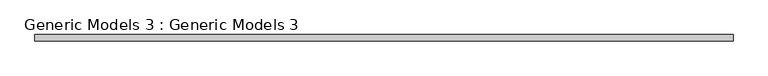
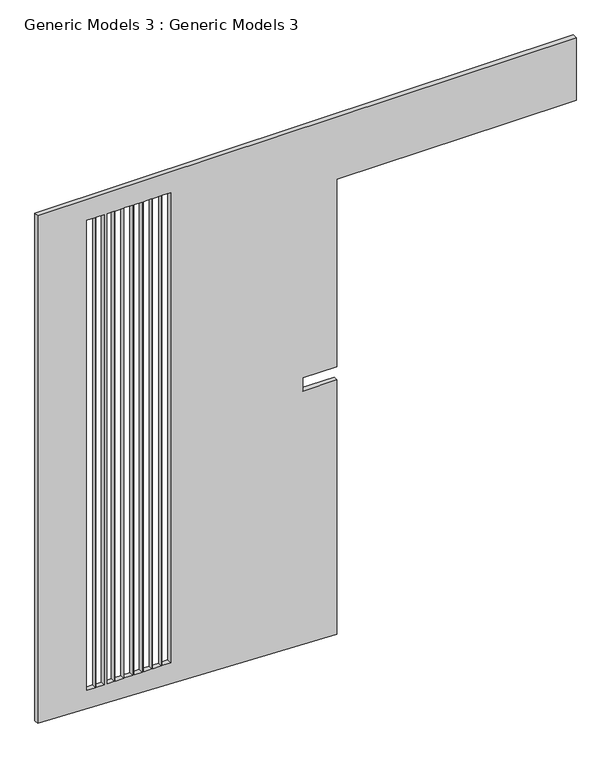
"""IFC4 building model written with IfcOpenShell, lengths in millimetres: proxy geometry, Generic Models 3 : Generic Models 3."""

from ifc_helpers import new_model, si_unit, frame, origin, place, context, project, spatial, polyline, outline, extrude, source, transform, mapped, element, save


def generic_models_3_generic_models_3_c928dfbd(model_context):
    return source(origin(), model_context, "Body", "SweptSolid", [
        extrude(outline(polyline([(8534.4, -2766.2781265), (8534.4, -937.4781265), (8534.4, -188.1781265), (9245.6, -188.1781265), (9245.6, -5990.8517085), (3465.4488588, -5990.8517085), (3352.8, -2766.2781265), (6248.4, -2766.2781265), (6248.4, -3134.5781265), (6400.8, -3134.5781265), (6400.8, -2766.2781265), (8534.4, -2766.2781265)]), holes=[polyline([(9008.4868285, -5369.7781265), (3653.3011148, -5369.7781265), (3653.3011148, -5461.3387619), (9008.4868285, -5461.3387619), (9008.4868285, -5369.7781265)]), polyline([(9008.4868285, -5275.2513777), (3653.3011148, -5275.2513777), (3653.3011148, -5359.7387619), (9008.4868285, -5359.7387619), (9008.4868285, -5275.2513777)]), polyline([(9008.4868285, -5166.5781265), (3653.3011148, -5166.5781265), (3653.3011148, -5242.7781265), (9008.4868285, -5242.7781265), (9008.4868285, -5166.5781265)]), polyline([(9008.4868285, -5064.9781265), (3653.3011148, -5064.9781265), (3653.3011148, -5156.5387619), (9008.4868285, -5156.5387619), (9008.4868285, -5064.9781265)]), polyline([(9008.4868285, -4966.4555102), (3653.3011148, -4966.4555102), (3653.3011148, -5054.9387619), (9008.4868285, -5054.9387619), (9008.4868285, -4966.4555102)]), polyline([(9008.4868285, -4865.3336422), (3653.3011148, -4865.3336422), (3653.3011148, -4951.2018509), (9008.4868285, -4951.2018509), (9008.4868285, -4865.3336422)]), polyline([(9008.4868285, -4760.1781265), (3653.3011148, -4760.1781265), (3653.3011148, -4849.0781265), (9008.4868285, -4849.0781265), (9008.4868285, -4760.1781265)]), polyline([(9008.4868285, -4658.5781265), (3653.3011148, -4658.5781265), (3653.3011148, -4750.1387619), (9008.4868285, -4750.1387619), (9008.4868285, -4658.5781265)]), polyline([(9008.4868285, -4556.9781265), (3653.3011148, -4556.9781265), (3653.3011148, -4648.5387619), (9008.4868285, -4648.5387619), (9008.4868285, -4556.9781265)])]), frame((0.0, -4440.0142532, 0.0), z_axis=(0.0, 1.0, 0.0), x_axis=(0.0, 0.0, 1.0)), (0.0, 0.0, 1.0), 50.8),
    ])


if __name__ == "__main__":
    model = new_model("IFC4")
    model_context = context("Model", 3, world=origin())
    ifc_project = project(units=[si_unit("LENGTHUNIT", "METRE", prefix="MILLI")], contexts=[model_context])
    site = spatial("IfcSite", under=ifc_project)
    building = spatial("IfcBuilding", under=site)
    placement = place(None, origin())
    generic_models_3_generic_models_3_shape = generic_models_3_generic_models_3_c928dfbd(model_context)
    element("IfcBuildingElementProxy", 1, Name="Generic Models 3 : Generic Models 3", ObjectType="Generic Models 3 : Generic Models 3", at=placement, inside=building, context=model_context, shape_type="MappedRepresentation", body=[
        mapped(generic_models_3_generic_models_3_shape, transform((0.0, 0.0, 0.0), x_axis=(1.0, 0.0, 0.0), y_axis=(0.0, 1.0, 0.0), z_axis=(0.0, 0.0, 1.0))),
    ])
    save(model, "model.ifc")
